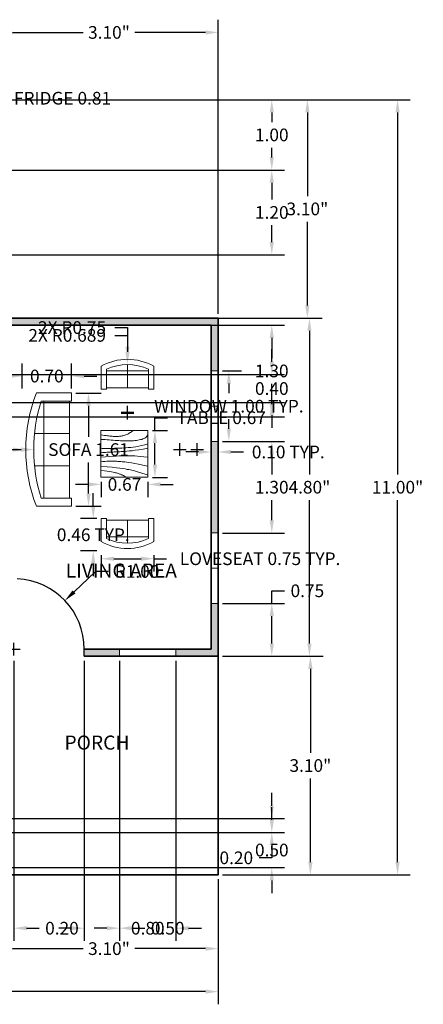
# Model space of a CAD drawing. Units: metres. Extents: x -1.9 to 13.1, y 0.9 to 14.8.
# Tile 7 of 7: x 7.4 to 13.1, y 0.9 to 14.8. Entities that reach past the tile are written whole.
import ezdxf

# ---------------------------------------------------------------- set-up
doc = ezdxf.new("R2010")
doc.units = ezdxf.units.M
doc.header["$MEASUREMENT"] = 0
for name, color, linetype, lineweight in [('A-ANNO-DIMS', 2, 'Continuous', 13), ('A-AREA-IDEN', 7, 'Continuous', 25), ('A-DOOR', 3, 'Continuous', 25), ('A-FURN', 8, 'Continuous', 18), ('A-GLAZ', 4, 'Continuous', 18), ('A-WALL', 7, 'Continuous', 35), ('A-WALL-PATT', 252, 'Continuous', 13)]:
    doc.layers.add(name, color=color, linetype=linetype, lineweight=lineweight)
doc.styles.get("Standard").update_dxf_attribs({"font": 'arial.ttf'})
doc.dimstyles.get("Standard").update_dxf_attribs({"dimtxt": 0.18, "dimasz": 0.18, "dimexe": 0.18, "dimexo": 0.0625, "dimgap": 0.09, "dimtad": 0, "dimtih": 1, "dimtoh": 1, "dimzin": 0, "dimdsep": 46, "dimlunit": 3, "dimtxsty": 'Standard', "dimcen": 0.09, "dimadec": 0, "dimazin": 0, "dimtfac": 1, "dimtofl": 0, "dimtmove": 0, "dimatfit": 3, "dimfxl": 1, "dimtolj": 1, "dimtzin": 0, "dimarcsym": 0})

# ---------------------------------------------------------------- blocks, each defined once
blk = doc.blocks.new('Table - Square Woodgrain 42 x 42 in.')
blk.add_line((0, -42), (42, -42))
for points in [[(0, -4), (1.704, -4.2172), (3.2358, -4.4188), (4.615, -4.604), (5.8615, -4.7721), (6.9951, -4.9224), (8.0357, -5.0541), (9.0031, -5.1667), (9.9171, -5.2594), (10.7951, -5.3316), (11.6445, -5.3836), (12.4702, -5.4157), (13.277, -5.4283), (14.0698, -5.4217), (14.8535, -5.3964), (15.6331, -5.3526), (16.4133, -5.2908), (17.1986, -5.2103), (17.9913, -5.1062), (18.793, -4.9727), (19.6056, -4.8038), (20.4307, -4.5937), (21.2701, -4.3365), (22.1256, -4.0262), (22.9989, -3.6571), (23.888, -3.2272), (24.7756, -2.7516), (25.6408, -2.2491), (26.4624, -1.7387), (27.2195, -1.2395), (27.891, -0.7703), (28.456, -0.3501), (28.8934, 0.002)], [(0, -42), (0, 0), (42, 0), (42, -42)], [(0, -8), (1.8203, -8.1001), (3.6741, -8.2149), (5.5411, -8.3408), (7.4011, -8.4741), (9.2339, -8.6112), (11.0193, -8.7484), (12.7371, -8.8821), (14.3671, -9.0086), (15.8954, -9.1246), (17.3337, -9.2278), (18.6997, -9.3159), (20.0116, -9.387), (21.2871, -9.4389), (22.5442, -9.4696), (23.8008, -9.477), (25.0749, -9.459), (26.3791, -9.4137), (27.7049, -9.3403), (29.0383, -9.2382), (30.3655, -9.1068), (31.6728, -8.9455), (32.9461, -8.7535), (34.1717, -8.5304), (35.3358, -8.2756), (36.4268, -7.9863), (37.443, -7.6521), (38.3849, -7.2603), (39.253, -6.7986), (40.048, -6.2542), (40.7705, -5.6147), (41.421, -4.8674), (42, -4)], [(42, -12), (39.1784, -12.8621), (36.4519, -13.5654), (33.8246, -14.1294), (31.3004, -14.5731), (28.8832, -14.9161), (26.577, -15.1775), (24.3858, -15.3768), (22.3136, -15.5332), (20.3622, -15.6632), (18.5254, -15.7718), (16.7947, -15.8612), (15.1618, -15.9338), (13.6183, -15.9916), (12.1558, -16.0369), (10.7659, -16.0718), (9.4403, -16.0987), (8.1703, -16.1191), (6.9461, -16.1325), (5.7577, -16.1377), (4.595, -16.1335), (3.4479, -16.1188), (2.3064, -16.0924), (1.1604, -16.0532), (0, -16)], [(42, -16), (37.6529, -16.7365), (33.8802, -17.329), (30.6179, -17.7961), (27.8015, -18.1561), (25.3668, -18.4275), (23.2497, -18.6288), (21.3859, -18.7785), (19.7111, -18.8949), (18.1693, -18.9939), (16.7375, -19.0795), (15.401, -19.1534), (14.1449, -19.217), (12.9544, -19.2717), (11.8148, -19.3191), (10.7113, -19.3606), (9.6291, -19.3976), (8.5534, -19.4323), (7.47, -19.4689), (6.3643, -19.5122), (5.222, -19.5672), (4.0288, -19.6386), (2.7703, -19.7313), (1.4321, -19.8501), (0, -20)], [(0, -24), (3.9243, -23.6805), (7.4766, -23.4138), (10.6891, -23.1954), (13.5943, -23.0205), (16.2247, -22.8847), (18.6125, -22.7832), (20.7903, -22.7116), (22.7903, -22.6651), (24.6563, -22.642), (26.4764, -22.6507), (28.35, -22.7024), (30.3766, -22.8084), (32.6555, -22.98), (35.2861, -23.2283), (38.3678, -23.5645), (42, -24)], [(42, -32), (37.392, -31.017), (33.4585, -30.2231), (30.1291, -29.5949), (27.3334, -29.109), (25.0009, -28.742), (23.0612, -28.4707), (21.4439, -28.2716), (20.0786, -28.1215), (18.8998, -28.0002), (17.8609, -27.9014), (16.9206, -27.8219), (16.0371, -27.7588), (15.1691, -27.709), (14.2748, -27.6693), (13.3128, -27.6368), (12.2415, -27.6083), (11.0295, -27.5824), (9.6867, -27.5643), (8.233, -27.5608), (6.6884, -27.5787), (5.0728, -27.6248), (3.4062, -27.7058), (1.7086, -27.8286), (0, -28)], [(0, -32), (5.4026, -32.5358), (9.9494, -33.019), (13.7424, -33.4553), (16.8834, -33.8505), (19.4743, -34.2106), (21.6171, -34.5413), (23.4136, -34.8486), (24.9657, -35.1382), (26.3614, -35.4156), (27.6332, -35.6841), (28.7995, -35.9467), (29.8788, -36.2064), (30.8897, -36.4661), (31.8507, -36.7288), (32.7802, -36.9973), (33.6968, -37.2747), (34.6175, -37.5635), (35.5531, -37.8651), (36.5128, -38.1805), (37.506, -38.5108), (38.5421, -38.8568), (39.6302, -39.2197), (40.7797, -39.6004), (42, -40)], [(0, -36), (3.0098, -36.2857), (5.5354, -36.5643), (7.6368, -36.8359), (9.374, -37.1009), (10.807, -37.3597), (11.9957, -37.6126), (13.0002, -37.8599), (13.8804, -38.102), (14.6874, -38.3393), (15.4365, -38.5729), (16.1338, -38.8041), (16.7858, -39.0341), (17.3987, -39.264), (17.9787, -39.4952), (18.5322, -39.7288), (19.0655, -39.9662), (19.5832, -40.2081), (20.0842, -40.4544), (20.5657, -40.7046), (21.0249, -40.9581), (21.459, -41.2144), (21.8653, -41.4731), (22.2409, -41.7335), (22.5831, -41.9951)]]:
    blk.add_lwpolyline(points)
blk = doc.blocks.new('Sofa - Roundback 7 ft.')
for p, q in [((-12.00002, -32.4421), (-12.00003, -6.5971)), ((11.99997, -32.4421), (11.99998, -6.5971)), ((-36.000027, -34), (-36.000027, -11.4696)), ((-35.999844, -13.3819), (35.9998, -13.3819)), ((35.99998, -34), (35.99998, -11.4696)), ((-36.000027, -32.4421), (35.99998, -32.4421))]:
    blk.add_line(p, q)
for points in [[(-36.000027, -34), (-42.000027, -34), (-42.000027, -8)], [(41.99998, -8), (41.99998, -34), (35.99998, -34)]]:
    blk.add_lwpolyline(points)
for centre, radius, start, end in [((0, -114.25), 114.25, 68.43141, 111.5686), ((-0.00001, -127.1968), 121.1968, 72.72033, 107.2797)]:
    blk.add_arc(centre, radius, start, end)
blk = doc.blocks.new('Sofa - Roundback Loveseat 5 ft.')
for p, q in [((0, -32.44198), (0, -5.99998)), ((-24, -33.99998), (-24, -11.46958)), ((-23.9998, -13.38178), (23.99986, -13.38178)), ((24.00004, -33.99998), (24.00004, -11.46958)), ((-24, -32.44198), (24.00004, -32.44198))]:
    blk.add_line(p, q)
for points in [[(-24, -33.99998), (-30, -33.99998), (-30, -7.99998)], [(30.00004, -7.99998), (30.00004, -33.99998), (24.00004, -33.99998)]]:
    blk.add_lwpolyline(points)
for centre, radius, start, end in [((0, -60.24998), 60.24998, 60.13715, 119.8628), ((0, -61.38438), 55.38444, 64.32083, 115.6792)]:
    blk.add_arc(centre, radius, start, end)
blk = doc.blocks.new('*D11')
at = {"layer": 'A-ANNO-DIMS', "color": 0, "lineweight": -2, "transparency": 16777216}
for p, q in [((7.104, 2.634), (7.104, 1.467)), ((10.204, 2.634), (10.204, 1.467)), ((7.284, 1.647), (8.286, 1.647)), ((10.024, 1.647), (9.022, 1.647))]:
    blk.add_line(p, q, dxfattribs=at)
at = {"layer": 'A-ANNO-DIMS', "color": 0, "transparency": 16777216}
for points in [[(7.284, 1.677), (7.284, 1.617), (7.104, 1.647)], [(10.024, 1.677), (10.024, 1.617), (10.204, 1.647)]]:
    blk.add_solid(points, dxfattribs=at)
at = {"layer": 'Defpoints', "color": 0, "transparency": 16777216}
for p in [(7.104, 2.696), (10.204, 2.696), (10.204, 1.647)]:
    blk.add_point(p, dxfattribs=at)
at = {"layer": 'A-ANNO-DIMS', "color": 0, "transparency": 16777216, "insert": (8.654, 1.647), "char_height": 0.18, "attachment_point": 5}
blk.add_mtext('\\A1;3.10"', dxfattribs=at)
blk = doc.blocks.new('*D12')
at = {"layer": 'A-ANNO-DIMS', "color": 0, "lineweight": -2, "transparency": 16777216}
for p, q in [((1.204, 2.634), (1.204, 0.857)), ((10.204, 2.634), (10.204, 0.857)), ((1.384, 1.037), (5.336, 1.037)), ((10.024, 1.037), (6.072, 1.037))]:
    blk.add_line(p, q, dxfattribs=at)
at = {"layer": 'A-ANNO-DIMS', "color": 0, "transparency": 16777216}
for points in [[(1.384, 1.067), (1.384, 1.007), (1.204, 1.037)], [(10.024, 1.067), (10.024, 1.007), (10.204, 1.037)]]:
    blk.add_solid(points, dxfattribs=at)
at = {"layer": 'Defpoints', "color": 0, "transparency": 16777216}
for p in [(1.204, 2.696), (10.204, 2.696), (10.204, 1.037)]:
    blk.add_point(p, dxfattribs=at)
at = {"layer": 'A-ANNO-DIMS', "color": 0, "transparency": 16777216, "insert": (5.704, 1.037), "char_height": 0.18, "attachment_point": 5}
blk.add_mtext('\\A1;9.00"', dxfattribs=at)
blk = doc.blocks.new('*D13')
at = {"layer": 'A-ANNO-DIMS', "color": 0, "lineweight": -2, "transparency": 16777216}
for p, q in [((7.166, 13.696), (12.927, 13.696)), ((12.747, 13.516), (12.747, 8.378)), ((12.747, 2.876), (12.747, 8.014)), ((10.266, 2.696), (12.927, 2.696))]:
    blk.add_line(p, q, dxfattribs=at)
at = {"layer": 'A-ANNO-DIMS', "color": 0, "transparency": 16777216}
for points in [[(12.717, 13.516), (12.777, 13.516), (12.747, 13.696)], [(12.717, 2.876), (12.777, 2.876), (12.747, 2.696)]]:
    blk.add_solid(points, dxfattribs=at)
at = {"layer": 'Defpoints', "color": 0, "transparency": 16777216}
for p in [(7.104, 13.696), (12.747, 13.696), (10.204, 2.696)]:
    blk.add_point(p, dxfattribs=at)
at = {"layer": 'A-ANNO-DIMS', "color": 0, "transparency": 16777216, "insert": (12.747, 8.196), "char_height": 0.18, "attachment_point": 5}
blk.add_mtext('\\A1;11.00"', dxfattribs=at)
blk = doc.blocks.new('*D14')
at = {"layer": 'A-ANNO-DIMS', "color": 0, "lineweight": -2, "transparency": 16777216}
for p, q in [((10.266, 5.796), (11.691, 5.796)), ((11.511, 5.616), (11.511, 4.428)), ((11.511, 2.876), (11.511, 4.064)), ((10.266, 2.696), (11.691, 2.696))]:
    blk.add_line(p, q, dxfattribs=at)
at = {"layer": 'A-ANNO-DIMS', "color": 0, "transparency": 16777216}
for points in [[(11.481, 5.616), (11.541, 5.616), (11.511, 5.796)], [(11.481, 2.876), (11.541, 2.876), (11.511, 2.696)]]:
    blk.add_solid(points, dxfattribs=at)
at = {"layer": 'Defpoints', "color": 0, "transparency": 16777216}
for p in [(10.204, 5.796), (11.511, 5.796), (10.204, 2.696)]:
    blk.add_point(p, dxfattribs=at)
at = {"layer": 'A-ANNO-DIMS', "color": 0, "transparency": 16777216, "insert": (11.511, 4.246), "char_height": 0.18, "attachment_point": 5}
blk.add_mtext('\\A1;3.10"', dxfattribs=at)
blk = doc.blocks.new('*D15')
at = {"layer": 'A-ANNO-DIMS', "color": 0, "lineweight": -2, "transparency": 16777216}
for p, q in [((10.266, 10.596), (11.677, 10.596)), ((11.497, 10.416), (11.497, 8.378)), ((11.497, 5.976), (11.497, 8.014)), ((10.266, 5.796), (11.677, 5.796))]:
    blk.add_line(p, q, dxfattribs=at)
at = {"layer": 'A-ANNO-DIMS', "color": 0, "transparency": 16777216}
for points in [[(11.467, 10.416), (11.527, 10.416), (11.497, 10.596)], [(11.467, 5.976), (11.527, 5.976), (11.497, 5.796)]]:
    blk.add_solid(points, dxfattribs=at)
at = {"layer": 'Defpoints', "color": 0, "transparency": 16777216}
for p in [(10.204, 10.596), (11.497, 10.596), (10.204, 5.796)]:
    blk.add_point(p, dxfattribs=at)
at = {"layer": 'A-ANNO-DIMS', "color": 0, "transparency": 16777216, "insert": (11.497, 8.196), "char_height": 0.18, "attachment_point": 5}
blk.add_mtext('\\A1;4.80"', dxfattribs=at)
blk = doc.blocks.new('*D16')
at = {"layer": 'A-ANNO-DIMS', "color": 0, "lineweight": -2, "transparency": 16777216}
for p, q in [((7.166, 13.696), (11.648, 13.696)), ((11.468, 13.516), (11.468, 12.328)), ((11.468, 10.776), (11.468, 11.964)), ((7.166, 10.596), (11.648, 10.596))]:
    blk.add_line(p, q, dxfattribs=at)
at = {"layer": 'A-ANNO-DIMS', "color": 0, "transparency": 16777216}
for points in [[(11.438, 13.516), (11.498, 13.516), (11.468, 13.696)], [(11.438, 10.776), (11.498, 10.776), (11.468, 10.596)]]:
    blk.add_solid(points, dxfattribs=at)
at = {"layer": 'Defpoints', "color": 0, "transparency": 16777216}
for p in [(7.104, 13.696), (11.468, 13.696), (7.104, 10.596)]:
    blk.add_point(p, dxfattribs=at)
at = {"layer": 'A-ANNO-DIMS', "color": 0, "transparency": 16777216, "insert": (11.468, 12.146), "char_height": 0.18, "attachment_point": 5}
blk.add_mtext('\\A1;3.10"', dxfattribs=at)
blk = doc.blocks.new('*D17')
at = {"layer": 'A-ANNO-DIMS', "color": 0, "lineweight": -2, "transparency": 16777216}
for p, q in [((7.104, 13.759), (7.104, 14.831)), ((10.204, 10.659), (10.204, 14.831)), ((7.284, 14.651), (8.286, 14.651)), ((10.024, 14.651), (9.022, 14.651))]:
    blk.add_line(p, q, dxfattribs=at)
at = {"layer": 'A-ANNO-DIMS', "color": 0, "transparency": 16777216}
for points in [[(7.284, 14.681), (7.284, 14.621), (7.104, 14.651)], [(10.024, 14.681), (10.024, 14.621), (10.204, 14.651)]]:
    blk.add_solid(points, dxfattribs=at)
at = {"layer": 'Defpoints', "color": 0, "transparency": 16777216}
for p in [(7.104, 14.651), (7.104, 13.696), (10.204, 10.596)]:
    blk.add_point(p, dxfattribs=at)
at = {"layer": 'A-ANNO-DIMS', "color": 0, "transparency": 16777216, "insert": (8.654, 14.651), "char_height": 0.18, "attachment_point": 5}
blk.add_mtext('\\A1;3.10"', dxfattribs=at)
blk = doc.blocks.new('WIN-1000')
for p, q in [((0.1, 1), (0, 1)), ((0.1, 0.5), (0, 0.5)), ((0.1, 0), (0, 0))]:
    blk.add_line(p, q)
blk = doc.blocks.new('*D28')
at = {"layer": 'A-ANNO-DIMS', "color": 0, "lineweight": -2, "transparency": 16777216}
for p, q in [((10.266, 9.846), (10.534, 9.846)), ((10.354, 9.666), (10.354, 9.53)), ((10.354, 9.026), (10.354, 9.163)), ((10.266, 8.846), (10.534, 8.846))]:
    blk.add_line(p, q, dxfattribs=at)
at = {"layer": 'A-ANNO-DIMS', "color": 0, "transparency": 16777216}
for points in [[(10.324, 9.666), (10.384, 9.666), (10.354, 9.846)], [(10.324, 9.026), (10.384, 9.026), (10.354, 8.846)]]:
    blk.add_solid(points, dxfattribs=at)
at = {"layer": 'Defpoints', "color": 0, "transparency": 16777216}
for p in [(10.204, 9.846), (10.354, 9.846), (10.204, 8.846)]:
    blk.add_point(p, dxfattribs=at)
at = {"layer": 'A-ANNO-DIMS', "color": 0, "transparency": 16777216, "insert": (10.354, 9.346), "char_height": 0.18, "attachment_point": 5}
blk.add_mtext('\\A1;WINDOW 1.00 TYP.', dxfattribs=at)
blk = doc.blocks.new('*D29')
at = {"layer": 'A-ANNO-DIMS', "color": 0, "lineweight": -2, "transparency": 16777216}
for p, q in [((9.924, 8.696), (9.744, 8.696)), ((10.104, 8.784), (10.104, 8.516)), ((10.204, 8.784), (10.204, 8.516)), ((10.384, 8.696), (10.564, 8.696))]:
    blk.add_line(p, q, dxfattribs=at)
at = {"layer": 'A-ANNO-DIMS', "color": 0, "transparency": 16777216}
for points in [[(9.924, 8.726), (9.924, 8.666), (10.104, 8.696)], [(10.384, 8.726), (10.384, 8.666), (10.204, 8.696)]]:
    blk.add_solid(points, dxfattribs=at)
at = {"layer": 'Defpoints', "color": 0, "transparency": 16777216}
for p in [(10.104, 8.846), (10.204, 8.846), (10.204, 8.696)]:
    blk.add_point(p, dxfattribs=at)
at = {"layer": 'A-ANNO-DIMS', "color": 0, "transparency": 16777216, "insert": (11.197, 8.696), "char_height": 0.18, "attachment_point": 5}
blk.add_mtext('\\A1;0.10 TYP.', dxfattribs=at)
blk = doc.blocks.new('*D38')
at = {"layer": 'A-ANNO-DIMS', "color": 0, "lineweight": -2, "transparency": 16777216}
for p, q in [((8.543, 7.231), (8.543, 7.001)), ((8.723, 7.181), (9.11, 7.181)), ((9.29, 7.231), (9.29, 7.001)), ((9.29, 7.181), (9.47, 7.181))]:
    blk.add_line(p, q, dxfattribs=at)
at = {"layer": 'A-ANNO-DIMS', "color": 0, "transparency": 16777216}
for points in [[(8.723, 7.211), (8.723, 7.151), (8.543, 7.181)], [(9.11, 7.211), (9.11, 7.151), (9.29, 7.181)]]:
    blk.add_solid(points, dxfattribs=at)
at = {"layer": 'Defpoints', "color": 0, "transparency": 16777216}
for p in [(8.543, 7.293), (9.29, 7.293), (9.29, 7.181)]:
    blk.add_point(p, dxfattribs=at)
at = {"layer": 'A-ANNO-DIMS', "color": 0, "transparency": 16777216, "insert": (10.797, 7.181), "char_height": 0.18, "attachment_point": 5}
blk.add_mtext('\\A1;LOVESEAT 0.75 TYP.', dxfattribs=at)
blk = doc.blocks.new('*D39')
at = {"layer": 'A-ANNO-DIMS', "color": 0, "lineweight": -2, "transparency": 16777216}
for p, q in [((8.431, 7.93), (8.431, 8.11)), ((8.481, 7.75), (8.251, 7.75)), ((8.481, 7.293), (8.251, 7.293)), ((8.431, 7.113), (8.431, 6.933))]:
    blk.add_line(p, q, dxfattribs=at)
at = {"layer": 'A-ANNO-DIMS', "color": 0, "transparency": 16777216}
for points in [[(8.401, 7.93), (8.461, 7.93), (8.431, 7.75)], [(8.401, 7.113), (8.461, 7.113), (8.431, 7.293)]]:
    blk.add_solid(points, dxfattribs=at)
at = {"layer": 'Defpoints', "color": 0, "transparency": 16777216}
for p in [(8.543, 7.75), (8.431, 7.293), (8.543, 7.293)]:
    blk.add_point(p, dxfattribs=at)
at = {"layer": 'A-ANNO-DIMS', "color": 0, "transparency": 16777216, "insert": (8.431, 7.521), "char_height": 0.18, "attachment_point": 5}
blk.add_mtext('\\A1;0.46 TYP.', dxfattribs=at)
blk = doc.blocks.new('*D40')
at = {"layer": 'A-ANNO-DIMS', "color": 0, "lineweight": -2, "transparency": 16777216}
for p, q in [((9.306, 9.002), (9.306, 9.182)), ((9.306, 9.182), (9.486, 9.182)), ((9.269, 9.002), (9.486, 9.002)), ((9.306, 8.516), (9.306, 8.822)), ((9.269, 8.336), (9.486, 8.336))]:
    blk.add_line(p, q, dxfattribs=at)
at = {"layer": 'A-ANNO-DIMS', "color": 0, "transparency": 16777216}
for points in [[(9.276, 8.822), (9.336, 8.822), (9.306, 9.002)], [(9.276, 8.516), (9.336, 8.516), (9.306, 8.336)]]:
    blk.add_solid(points, dxfattribs=at)
at = {"layer": 'Defpoints', "color": 0, "transparency": 16777216}
for p in [(9.206, 9.002), (9.306, 9.002), (9.206, 8.336)]:
    blk.add_point(p, dxfattribs=at)
at = {"layer": 'A-ANNO-DIMS', "color": 0, "transparency": 16777216, "insert": (10.246, 9.182), "char_height": 0.18, "attachment_point": 5}
blk.add_mtext('\\A1;TABLE 0.67', dxfattribs=at)
blk = doc.blocks.new('*D41')
at = {"layer": 'A-ANNO-DIMS', "color": 0, "lineweight": -2, "transparency": 16777216}
for p, q in [((8.541, 8.274), (8.541, 8.056)), ((9.206, 8.274), (9.206, 8.056)), ((8.361, 8.236), (8.181, 8.236)), ((9.386, 8.236), (9.566, 8.236))]:
    blk.add_line(p, q, dxfattribs=at)
at = {"layer": 'A-ANNO-DIMS', "color": 0, "transparency": 16777216}
for points in [[(8.361, 8.266), (8.361, 8.206), (8.541, 8.236)], [(9.386, 8.266), (9.386, 8.206), (9.206, 8.236)]]:
    blk.add_solid(points, dxfattribs=at)
at = {"layer": 'Defpoints', "color": 0, "transparency": 16777216}
for p in [(8.541, 8.336), (9.206, 8.336), (9.206, 8.236)]:
    blk.add_point(p, dxfattribs=at)
at = {"layer": 'A-ANNO-DIMS', "color": 0, "transparency": 16777216, "insert": (8.874, 8.236), "char_height": 0.18, "attachment_point": 5}
blk.add_mtext('\\A1;0.67', dxfattribs=at)
blk = doc.blocks.new('*D42')
at = {"layer": 'A-ANNO-DIMS', "color": 0, "lineweight": -2, "transparency": 16777216}
for p, q in [((8.185, 9.533), (8.544, 9.533)), ((8.364, 9.353), (8.364, 8.913)), ((8.364, 8.106), (8.364, 8.547)), ((8.185, 7.926), (8.544, 7.926))]:
    blk.add_line(p, q, dxfattribs=at)
at = {"layer": 'A-ANNO-DIMS', "color": 0, "transparency": 16777216}
for points in [[(8.334, 9.353), (8.394, 9.353), (8.364, 9.533)], [(8.334, 8.106), (8.394, 8.106), (8.364, 7.926)]]:
    blk.add_solid(points, dxfattribs=at)
at = {"layer": 'Defpoints', "color": 0, "transparency": 16777216}
for p in [(8.123, 9.533), (8.364, 9.533), (8.123, 7.926)]:
    blk.add_point(p, dxfattribs=at)
at = {"layer": 'A-ANNO-DIMS', "color": 0, "transparency": 16777216, "insert": (8.364, 8.73), "char_height": 0.18, "attachment_point": 5}
blk.add_mtext('\\A1;SOFA 1.61', dxfattribs=at)
blk = doc.blocks.new('*D43')
at = {"layer": 'A-ANNO-DIMS', "color": 0, "lineweight": -2, "transparency": 16777216}
for p, q in [((7.421, 9.596), (7.421, 9.954)), ((8.123, 9.596), (8.123, 9.954)), ((7.241, 9.774), (7.061, 9.774)), ((8.303, 9.774), (8.483, 9.774))]:
    blk.add_line(p, q, dxfattribs=at)
at = {"layer": 'A-ANNO-DIMS', "color": 0, "transparency": 16777216}
for points in [[(7.241, 9.804), (7.241, 9.744), (7.421, 9.774)], [(8.303, 9.804), (8.303, 9.744), (8.123, 9.774)]]:
    blk.add_solid(points, dxfattribs=at)
at = {"layer": 'Defpoints', "color": 0, "transparency": 16777216}
for p in [(7.421, 9.774), (7.421, 9.533), (8.123, 9.533)]:
    blk.add_point(p, dxfattribs=at)
at = {"layer": 'A-ANNO-DIMS', "color": 0, "transparency": 16777216, "insert": (7.772, 9.774), "char_height": 0.18, "attachment_point": 5}
blk.add_mtext('\\A1;0.70', dxfattribs=at)
blk = doc.blocks.new('*D46')
at = {"layer": 'A-ANNO-DIMS', "color": 0, "lineweight": -2, "transparency": 16777216}
for p, q in [((6.197, 13.659), (6.197, 13.897)), ((7.004, 13.659), (7.004, 13.897)), ((6.377, 13.717), (6.824, 13.717)), ((7.004, 13.717), (7.184, 13.717))]:
    blk.add_line(p, q, dxfattribs=at)
at = {"layer": 'A-ANNO-DIMS', "color": 0, "transparency": 16777216}
for points in [[(6.377, 13.747), (6.377, 13.687), (6.197, 13.717)], [(6.824, 13.747), (6.824, 13.687), (7.004, 13.717)]]:
    blk.add_solid(points, dxfattribs=at)
at = {"layer": 'Defpoints', "color": 0, "transparency": 16777216}
for p in [(7.004, 13.717), (6.197, 13.596), (7.004, 13.596)]:
    blk.add_point(p, dxfattribs=at)
at = {"layer": 'A-ANNO-DIMS', "color": 0, "transparency": 16777216, "insert": (7.995, 13.717), "char_height": 0.18, "attachment_point": 5}
blk.add_mtext('\\A1;FRIDGE 0.81', dxfattribs=at)
blk = doc.blocks.new('*D55')
at = {"layer": 'A-ANNO-DIMS', "color": 0, "lineweight": -2, "transparency": 16777216}
for p, q in [((10.963, 6.546), (10.963, 6.726)), ((10.963, 6.726), (11.143, 6.726)), ((10.266, 6.546), (11.143, 6.546)), ((10.963, 5.976), (10.963, 6.366)), ((10.266, 5.796), (11.143, 5.796))]:
    blk.add_line(p, q, dxfattribs=at)
at = {"layer": 'A-ANNO-DIMS', "color": 0, "transparency": 16777216}
for points in [[(10.933, 6.366), (10.993, 6.366), (10.963, 6.546)], [(10.933, 5.976), (10.993, 5.976), (10.963, 5.796)]]:
    blk.add_solid(points, dxfattribs=at)
at = {"layer": 'Defpoints', "color": 0, "transparency": 16777216}
for p in [(10.204, 6.546), (10.963, 6.546), (10.204, 5.796)]:
    blk.add_point(p, dxfattribs=at)
at = {"layer": 'A-ANNO-DIMS', "color": 0, "transparency": 16777216, "insert": (11.468, 6.726), "char_height": 0.18, "attachment_point": 5}
blk.add_mtext('\\A1;0.75', dxfattribs=at)
blk = doc.blocks.new('*D56')
at = {"layer": 'A-ANNO-DIMS', "color": 0, "lineweight": -2, "transparency": 16777216}
for p, q in [((10.266, 8.846), (11.143, 8.846)), ((10.963, 8.666), (10.963, 8.378)), ((10.963, 7.726), (10.963, 8.014)), ((10.266, 7.546), (11.143, 7.546))]:
    blk.add_line(p, q, dxfattribs=at)
at = {"layer": 'A-ANNO-DIMS', "color": 0, "transparency": 16777216}
for points in [[(10.933, 8.666), (10.993, 8.666), (10.963, 8.846)], [(10.933, 7.726), (10.993, 7.726), (10.963, 7.546)]]:
    blk.add_solid(points, dxfattribs=at)
at = {"layer": 'Defpoints', "color": 0, "transparency": 16777216}
for p in [(10.204, 8.846), (10.963, 8.846), (10.204, 7.546)]:
    blk.add_point(p, dxfattribs=at)
at = {"layer": 'A-ANNO-DIMS', "color": 0, "transparency": 16777216, "insert": (10.963, 8.196), "char_height": 0.18, "attachment_point": 5}
blk.add_mtext('\\A1;1.30', dxfattribs=at)
blk = doc.blocks.new('*D57')
at = {"layer": 'A-ANNO-DIMS', "color": 0, "lineweight": -2, "transparency": 16777216}
for p, q in [((8.304, 5.734), (8.304, 1.757)), ((8.804, 5.734), (8.804, 1.757)), ((8.124, 1.937), (7.944, 1.937)), ((8.984, 1.937), (9.164, 1.937))]:
    blk.add_line(p, q, dxfattribs=at)
at = {"layer": 'A-ANNO-DIMS', "color": 0, "transparency": 16777216}
for points in [[(8.124, 1.967), (8.124, 1.907), (8.304, 1.937)], [(8.984, 1.967), (8.984, 1.907), (8.804, 1.937)]]:
    blk.add_solid(points, dxfattribs=at)
at = {"layer": 'Defpoints', "color": 0, "transparency": 16777216}
for p in [(8.304, 5.796), (8.804, 5.796), (8.804, 1.937)]:
    blk.add_point(p, dxfattribs=at)
at = {"layer": 'A-ANNO-DIMS', "color": 0, "transparency": 16777216, "insert": (9.487, 1.937), "char_height": 0.18, "attachment_point": 5}
blk.add_mtext('\\A1;0.50', dxfattribs=at)
blk = doc.blocks.new('*D58')
at = {"layer": 'A-ANNO-DIMS', "color": 0, "lineweight": -2, "transparency": 16777216}
for p, q in [((8.803847, 5.733878), (8.803847, 1.756878)), ((9.603847, 5.733878), (9.603847, 1.756878)), ((8.623847, 1.936878), (8.443847, 1.936878)), ((9.783847, 1.936878), (9.963847, 1.936878))]:
    blk.add_line(p, q, dxfattribs=at)
at = {"layer": 'A-ANNO-DIMS', "color": 0, "transparency": 16777216}
for points in [[(8.623847, 1.966878), (8.623847, 1.906878), (8.803847, 1.936878)], [(9.783847, 1.966878), (9.783847, 1.906878), (9.603847, 1.936878)]]:
    blk.add_solid(points, dxfattribs=at)
at = {"layer": 'Defpoints', "color": 0, "transparency": 16777216}
for p in [(8.803847, 5.796378), (9.603847, 5.796378), (8.803847, 1.936878)]:
    blk.add_point(p, dxfattribs=at)
at = {"layer": 'A-ANNO-DIMS', "color": 0, "transparency": 16777216, "insert": (9.203847, 1.936878), "char_height": 0.18, "attachment_point": 5}
blk.add_mtext('\\A1;0.80', dxfattribs=at)
blk = doc.blocks.new('*D59')
at = {"layer": 'A-ANNO-DIMS', "color": 0, "lineweight": -2, "transparency": 16777216}
for p, q in [((7.104, 5.734), (7.104, 1.757)), ((7.304, 5.734), (7.304, 1.757)), ((6.924, 1.937), (6.744, 1.937)), ((7.484, 1.937), (7.664, 1.937))]:
    blk.add_line(p, q, dxfattribs=at)
at = {"layer": 'A-ANNO-DIMS', "color": 0, "transparency": 16777216}
for points in [[(6.924, 1.967), (6.924, 1.907), (7.104, 1.937)], [(7.484, 1.967), (7.484, 1.907), (7.304, 1.937)]]:
    blk.add_solid(points, dxfattribs=at)
at = {"layer": 'Defpoints', "color": 0, "transparency": 16777216}
for p in [(7.104, 5.796), (7.304, 5.796), (7.304, 1.937)]:
    blk.add_point(p, dxfattribs=at)
at = {"layer": 'A-ANNO-DIMS', "color": 0, "transparency": 16777216, "insert": (7.987, 1.937), "char_height": 0.18, "attachment_point": 5}
blk.add_mtext('\\A1;0.20', dxfattribs=at)
blk = doc.blocks.new('*D60')
at = {"layer": 'A-ANNO-DIMS', "color": 0, "lineweight": -2, "transparency": 16777216}
for p, q in [((7.166, 13.696), (11.143, 13.696)), ((10.963, 13.516), (10.963, 13.378)), ((10.963, 12.876), (10.963, 13.014)), ((7.166, 12.696), (11.143, 12.696))]:
    blk.add_line(p, q, dxfattribs=at)
at = {"layer": 'A-ANNO-DIMS', "color": 0, "transparency": 16777216}
for points in [[(10.933, 13.516), (10.993, 13.516), (10.963, 13.696)], [(10.933, 12.876), (10.993, 12.876), (10.963, 12.696)]]:
    blk.add_solid(points, dxfattribs=at)
at = {"layer": 'Defpoints', "color": 0, "transparency": 16777216}
for p in [(7.104, 13.696), (10.963, 13.696), (7.104, 12.696)]:
    blk.add_point(p, dxfattribs=at)
at = {"layer": 'A-ANNO-DIMS', "color": 0, "transparency": 16777216, "insert": (10.963, 13.196), "char_height": 0.18, "attachment_point": 5}
blk.add_mtext('\\A1;1.00', dxfattribs=at)
blk = doc.blocks.new('*D61')
at = {"layer": 'A-ANNO-DIMS', "color": 0, "lineweight": -2, "transparency": 16777216}
for p, q in [((7.166, 12.696), (11.143, 12.696)), ((10.963, 12.516), (10.963, 12.278)), ((10.963, 11.676), (10.963, 11.914)), ((7.166, 11.496), (11.143, 11.496))]:
    blk.add_line(p, q, dxfattribs=at)
at = {"layer": 'A-ANNO-DIMS', "color": 0, "transparency": 16777216}
for points in [[(10.933, 12.516), (10.993, 12.516), (10.963, 12.696)], [(10.933, 11.676), (10.993, 11.676), (10.963, 11.496)]]:
    blk.add_solid(points, dxfattribs=at)
at = {"layer": 'Defpoints', "color": 0, "transparency": 16777216}
for p in [(7.104, 12.696), (7.104, 11.496), (10.963, 11.496)]:
    blk.add_point(p, dxfattribs=at)
at = {"layer": 'A-ANNO-DIMS', "color": 0, "transparency": 16777216, "insert": (10.963, 12.096), "char_height": 0.18, "attachment_point": 5}
blk.add_mtext('\\A1;1.20', dxfattribs=at)
blk = doc.blocks.new('*D65')
at = {"layer": 'A-ANNO-DIMS', "color": 0, "lineweight": -2, "transparency": 16777216}
for p, q in [((10.963347, 9.976378), (10.963347, 10.156378)), ((2.966347, 9.796378), (11.143347, 9.796378)), ((2.966347, 9.396378), (11.143347, 9.396378)), ((10.963347, 9.216378), (10.963347, 9.036378))]:
    blk.add_line(p, q, dxfattribs=at)
at = {"layer": 'A-ANNO-DIMS', "color": 0, "transparency": 16777216}
for points in [[(10.933347, 9.976378), (10.993347, 9.976378), (10.963347, 9.796378)], [(10.933347, 9.216378), (10.993347, 9.216378), (10.963347, 9.396378)]]:
    blk.add_solid(points, dxfattribs=at)
at = {"layer": 'Defpoints', "color": 0, "transparency": 16777216}
for p in [(2.903847, 9.796378), (2.903847, 9.396378), (10.963347, 9.396378)]:
    blk.add_point(p, dxfattribs=at)
at = {"layer": 'A-ANNO-DIMS', "color": 0, "transparency": 16777216, "insert": (10.963347, 9.596378), "char_height": 0.18, "attachment_point": 5}
blk.add_mtext('\\A1;0.40', dxfattribs=at)
blk = doc.blocks.new('*D67')
at = {"layer": 'A-ANNO-DIMS', "color": 0, "lineweight": -2, "transparency": 16777216}
for p, q in [((10.963, 3.676), (10.963, 3.856)), ((7.066, 3.496), (11.143, 3.496)), ((7.066, 3.296), (11.143, 3.296)), ((10.963, 3.116), (10.963, 2.936)), ((10.963, 2.936), (10.783, 2.936))]:
    blk.add_line(p, q, dxfattribs=at)
at = {"layer": 'A-ANNO-DIMS', "color": 0, "transparency": 16777216}
for points in [[(10.933, 3.676), (10.993, 3.676), (10.963, 3.496)], [(10.933, 3.116), (10.993, 3.116), (10.963, 3.296)]]:
    blk.add_solid(points, dxfattribs=at)
at = {"layer": 'Defpoints', "color": 0, "transparency": 16777216}
for p in [(7.004, 3.496), (7.004, 3.296), (10.963, 3.296)]:
    blk.add_point(p, dxfattribs=at)
at = {"layer": 'A-ANNO-DIMS', "color": 0, "transparency": 16777216, "insert": (10.46, 2.936), "char_height": 0.18, "attachment_point": 5}
blk.add_mtext('\\A1;0.20', dxfattribs=at)
blk = doc.blocks.new('*D68')
at = {"layer": 'A-ANNO-DIMS', "color": 0, "lineweight": -2, "transparency": 16777216}
for p, q in [((10.963347, 3.476378), (10.963347, 3.656378)), ((7.066347, 3.296378), (11.143347, 3.296378)), ((7.066347, 2.796378), (11.143347, 2.796378)), ((10.963347, 2.616378), (10.963347, 2.436378))]:
    blk.add_line(p, q, dxfattribs=at)
at = {"layer": 'A-ANNO-DIMS', "color": 0, "transparency": 16777216}
for points in [[(10.933347, 3.476378), (10.993347, 3.476378), (10.963347, 3.296378)], [(10.933347, 2.616378), (10.993347, 2.616378), (10.963347, 2.796378)]]:
    blk.add_solid(points, dxfattribs=at)
at = {"layer": 'Defpoints', "color": 0, "transparency": 16777216}
for p in [(7.003847, 3.296378), (7.003847, 2.796378), (10.963347, 2.796378)]:
    blk.add_point(p, dxfattribs=at)
at = {"layer": 'A-ANNO-DIMS', "color": 0, "transparency": 16777216, "insert": (10.963347, 3.046378), "char_height": 0.18, "attachment_point": 5}
blk.add_mtext('\\A1;0.50', dxfattribs=at)
blk = doc.blocks.new('*D74')
at = {"layer": 'A-ANNO-DIMS', "color": 0, "lineweight": -2, "transparency": 16777216}
for p, q in [((7.166, 10.496), (11.143, 10.496)), ((10.963, 10.316), (10.963, 10.028)), ((10.963, 9.376), (10.963, 9.664)), ((7.166, 9.196), (11.143, 9.196))]:
    blk.add_line(p, q, dxfattribs=at)
at = {"layer": 'A-ANNO-DIMS', "color": 0, "transparency": 16777216}
for points in [[(10.933, 10.316), (10.993, 10.316), (10.963, 10.496)], [(10.933, 9.376), (10.993, 9.376), (10.963, 9.196)]]:
    blk.add_solid(points, dxfattribs=at)
at = {"layer": 'Defpoints', "color": 0, "transparency": 16777216}
for p in [(7.104, 10.496), (10.963, 10.496), (7.104, 9.196)]:
    blk.add_point(p, dxfattribs=at)
at = {"layer": 'A-ANNO-DIMS', "color": 0, "transparency": 16777216, "insert": (10.963, 9.846), "char_height": 0.18, "attachment_point": 5}
blk.add_mtext('\\A1;1.30', dxfattribs=at)
blk = doc.blocks.new('*D75')
at = {"layer": 'A-ANNO-DIMS', "color": 0, "lineweight": -2, "transparency": 16777216}
for p, q in [((8.464, 7), (8.159, 6.71)), ((8.644, 7), (8.464, 7)), ((7.213, 5.896), (7.393, 5.896)), ((7.303, 5.806), (7.303, 5.986))]:
    blk.add_line(p, q, dxfattribs=at)
at = {"layer": 'A-ANNO-DIMS', "color": 0, "transparency": 16777216}
blk.add_solid([(8.138, 6.732), (8.179, 6.689), (8.028, 6.586)], dxfattribs=at)
at = {"layer": 'Defpoints', "color": 0, "transparency": 16777216}
for p in [(8.028, 6.586), (7.303, 5.896)]:
    blk.add_point(p, dxfattribs=at)
at = {"layer": 'A-ANNO-DIMS', "color": 0, "transparency": 16777216, "insert": (9.053, 7), "char_height": 0.18, "attachment_point": 5}
blk.add_mtext('\\A1;R1.00', dxfattribs=at)
blk = doc.blocks.new('*D78')
at = {"layer": 'A-ANNO-DIMS', "color": 0, "lineweight": -2, "transparency": 16777216}
for p, q in [((9.906, 8.64), (9.906, 8.82)), ((6.196, 8.73), (7.407, 8.73)), ((9.816, 8.73), (9.996, 8.73))]:
    blk.add_line(p, q, dxfattribs=at)
at = {"layer": 'A-ANNO-DIMS', "color": 0, "transparency": 16777216}
blk.add_solid([(7.407, 8.76), (7.407, 8.7), (7.587, 8.73)], dxfattribs=at)
at = {"layer": 'Defpoints', "color": 0, "transparency": 16777216}
for p in [(7.587, 8.73), (9.906, 8.73)]:
    blk.add_point(p, dxfattribs=at)
at = {"layer": 'A-ANNO-DIMS', "color": 0, "transparency": 16777216, "insert": (5.787, 8.73), "char_height": 0.18, "attachment_point": 5}
blk.add_mtext('\\A1;R2.32', dxfattribs=at)
blk = doc.blocks.new('*D79')
at = {"layer": 'A-ANNO-DIMS', "color": 0, "lineweight": -2, "transparency": 16777216}
for p, q in [((9.658, 8.64), (9.658, 8.82)), ((6.161, 8.73), (7.292, 8.73)), ((9.568, 8.73), (9.748, 8.73))]:
    blk.add_line(p, q, dxfattribs=at)
at = {"layer": 'A-ANNO-DIMS', "color": 0, "transparency": 16777216}
blk.add_solid([(7.292, 8.76), (7.292, 8.7), (7.472, 8.73)], dxfattribs=at)
at = {"layer": 'Defpoints', "color": 0, "transparency": 16777216}
for p in [(7.472, 8.73), (9.658, 8.73)]:
    blk.add_point(p, dxfattribs=at)
at = {"layer": 'A-ANNO-DIMS', "color": 0, "transparency": 16777216, "insert": (5.751, 8.73), "char_height": 0.18, "attachment_point": 5}
blk.add_mtext('\\A1;R2.19', dxfattribs=at)
blk = doc.blocks.new('*D80')
at = {"layer": 'A-ANNO-DIMS', "color": 0, "lineweight": -2, "transparency": 16777216}
for p, q in [((8.736, 10.462), (8.916, 10.462)), ((8.916, 10.462), (8.916, 10.192)), ((8.826, 9.262), (9.006, 9.262)), ((8.916, 9.172), (8.916, 9.352))]:
    blk.add_line(p, q, dxfattribs=at)
at = {"layer": 'A-ANNO-DIMS', "color": 0, "transparency": 16777216}
blk.add_solid([(8.946, 10.192), (8.886, 10.192), (8.916, 10.012)], dxfattribs=at)
at = {"layer": 'Defpoints', "color": 0, "transparency": 16777216}
for p in [(8.916, 10.012), (8.916, 9.262)]:
    blk.add_point(p, dxfattribs=at)
at = {"layer": 'A-ANNO-DIMS', "color": 0, "transparency": 16777216, "insert": (8.13, 10.462), "char_height": 0.18, "attachment_point": 5}
blk.add_mtext('\\A1;2X R0.75', dxfattribs=at)
blk = doc.blocks.new('*D81')
at = {"layer": 'A-ANNO-DIMS', "color": 0, "lineweight": -2, "transparency": 16777216}
for p, q in [((8.736, 10.351), (8.916, 10.351)), ((8.916, 10.351), (8.916, 10.117)), ((8.826, 9.248), (9.006, 9.248)), ((8.916, 9.158), (8.916, 9.338))]:
    blk.add_line(p, q, dxfattribs=at)
at = {"layer": 'A-ANNO-DIMS', "color": 0, "transparency": 16777216}
blk.add_solid([(8.946, 10.117), (8.886, 10.117), (8.916, 9.937)], dxfattribs=at)
at = {"layer": 'Defpoints', "color": 0, "transparency": 16777216}
for p in [(8.916, 9.937), (8.916, 9.248)]:
    blk.add_point(p, dxfattribs=at)
at = {"layer": 'A-ANNO-DIMS', "color": 0, "transparency": 16777216, "insert": (8.061, 10.351), "char_height": 0.18, "attachment_point": 5}
blk.add_mtext('\\A1;2X R0.689', dxfattribs=at)

msp = doc.modelspace()

# ---------------------------------------------------------------- linework, layer by layer
at = {"layer": 'A-DOOR'}
msp.add_line((8.3038, 5.7964), (8.3038, 5.8964), dxfattribs=at)
msp.add_arc((7.3025, 5.8964), 1.0013, 0, 87.0624, dxfattribs=at)
at = {"layer": 'A-GLAZ'}
for p, q in [((8.8038, 5.7964), (8.8038, 5.8964)), ((9.6038, 5.7964), (9.6038, 5.8964))]:
    msp.add_line(p, q, dxfattribs=at)
at = {"layer": 'A-WALL'}
for p, q in [((10.2038, 10.5964), (7.1038, 10.5964)), ((10.1038, 10.4964), (7.1038, 10.4964)), ((10.1038, 5.8964), (10.1038, 10.4964)), ((8.3038, 5.8964), (10.1038, 5.8964)), ((8.3038, 5.7964), (10.2038, 5.7964))]:
    msp.add_line(p, q, dxfattribs=at)
msp.add_lwpolyline([(1.2038, 10.5964), (1.2038, 2.6964), (10.2038, 2.6964), (10.2038, 10.5964)], dxfattribs=at)
at = {"layer": 'A-WALL-PATT'}
for points in [[(7.1038, 10.5964), (7.1038, 10.4964), (10.2038, 10.5964), (10.1038, 10.4964)], [(10.2038, 10.5964), (10.1038, 10.4964), (10.2038, 9.8464), (10.1038, 9.8464)], [(10.2038, 8.8464), (10.1038, 8.8464), (10.2038, 7.5464), (10.1038, 7.5464)], [(10.2038, 6.5464), (10.1038, 6.5464), (10.2038, 5.7964), (10.1038, 5.8964)], [(8.3038, 5.8964), (8.3038, 5.7964), (8.8038, 5.8964), (8.8038, 5.7964)], [(10.2038, 5.7964), (10.1038, 5.8964), (9.6038, 5.7964), (9.6038, 5.8964)]]:
    msp.add_solid(points, dxfattribs=at)

# ---------------------------------------------------------------- block references
at = {"layer": 'A-FURN'}
for name, p, xscale, yscale, zscale in [('Sofa - Roundback Loveseat 5 ft.', (8.9163, 10.0119), 0.0124407899169528, 0.0124407899169528, 0.0124407899169528), ('Table - Square Woodgrain 42 x 42 in.', (8.5407, 9.0021), 0.0158519900897889, 0.0158519900897889, 0.0158519900897889)]:
    msp.add_blockref(name, p, dxfattribs=dict(at, xscale=xscale, yscale=yscale, zscale=zscale))
for name, p, xscale, yscale, zscale, rotation in [('Sofa - Roundback 7 ft.', (7.4724, 8.7299), 0.0191300875389889, 0.0191300875389889, 0.0191300875389889, 90), ('Sofa - Roundback Loveseat 5 ft.', (8.9163, 7.3266), -0.0124407899169528, 0.0124407899169528, 0.0124407899169528, 180)]:
    msp.add_blockref(name, p, dxfattribs=dict(at, xscale=xscale, yscale=yscale, zscale=zscale, rotation=rotation))
at = {"layer": 'A-GLAZ'}
for p in [(10.1038, 8.8464), (10.1038, 6.5464)]:
    msp.add_blockref('WIN-1000', p, dxfattribs=at)

# ---------------------------------------------------------------- texts
at = {"layer": 'A-AREA-IDEN', "char_height": 0.2, "attachment_point": 1}
for s, width, insert in [('LIVING AREA', 1.759091, (8.0405, 7.1125)), ('\\pxqc;PORCH', 1.033831, (7.9664, 4.6715))]:
    msp.add_mtext_dynamic_manual_height_columns(s, width=width, gutter_width=1, heights=[0], dxfattribs=dict(at, insert=insert))

# ---------------------------------------------------------------- dimensions: what is measured, and where the dimension line sits
at = {"layer": 'A-ANNO-DIMS'}
for base, p1, p2, override, picture, middle in [((7.1038, 14.6515), (10.2038, 10.5964), (7.1038, 13.6964), {"dimclrd": 0, "dimclre": 0, "dimclrt": 0}, '*D17', (8.6538, 14.6515)), ((9.2065, 8.2365), (8.5407, 8.3364), (9.2065, 8.3364), {"dimdec": 2, "dimlfac": 1, "dimrnd": 0, "dimzin": 0, "dimdsep": 46, "dimlunit": 2}, '*D41', (8.8736, 8.2365)), ((7.3038, 1.9369), (7.1038, 5.7964), (7.3038, 5.7964), {"dimdec": 2, "dimlfac": 1, "dimrnd": 0, "dimzin": 0, "dimdsep": 46, "dimlunit": 2}, '*D59', (7.9873, 1.9369)), ((8.8038, 1.9369), (8.3038, 5.7964), (8.8038, 5.7964), {"dimdec": 2, "dimlfac": 1, "dimrnd": 0, "dimzin": 0, "dimdsep": 46, "dimlunit": 2}, '*D57', (9.4873, 1.9369)), ((8.8038, 1.9369), (9.6038, 5.7964), (8.8038, 5.7964), {"dimdec": 2, "dimlfac": 1, "dimrnd": 0, "dimzin": 0, "dimdsep": 46, "dimlunit": 2}, '*D58', (9.2038, 1.9369)), ((10.2038, 1.0368), (1.2038, 2.6964), (10.2038, 2.6964), {"dimclrd": 0, "dimclre": 0, "dimclrt": 0}, '*D12', (5.7038, 1.0368)), ((10.2038, 1.647), (7.1038, 2.6964), (10.2038, 2.6964), {"dimclrd": 0, "dimclre": 0, "dimclrt": 0}, '*D11', (8.6538, 1.647))]:
    dim = msp.add_linear_dim(base=base, p1=p1, p2=p2, dimstyle='Standard', override=override, dxfattribs=at)
    dim.commit()
    dim.dimension.update_dxf_attribs({"geometry": picture, "text_midpoint": middle})
for base, p1, p2, text, picture, middle in [((7.0038, 13.7174), (6.197, 13.5964), (7.0038, 13.5964), 'FRIDGE <>', '*D46', (7.9951, 13.7174)), ((10.2038, 8.6964), (10.1038, 8.8464), (10.2038, 8.8464), '<> TYP.', '*D29', (11.1968, 8.6964)), ((9.2895, 7.1814), (8.5431, 7.2934), (9.2895, 7.2934), 'LOVESEAT <> TYP.', '*D38', (10.7972, 7.1814))]:
    dim = msp.add_linear_dim(base=base, p1=p1, p2=p2, text=text, dimstyle='Standard', override={"dimdec": 2, "dimlfac": 1, "dimrnd": 0, "dimzin": 0, "dimdsep": 46, "dimlunit": 2}, dxfattribs=at)
    dim.commit()
    dim.dimension.update_dxf_attribs({"geometry": picture, "text_midpoint": middle})
for base, p1, p2, angle, override, picture, middle in [((12.7472, 13.6964), (10.2038, 2.6964), (7.1038, 13.6964), 90, {"dimclrd": 0, "dimclre": 0, "dimclrt": 0}, '*D13', (12.7472, 8.1964)), ((11.4682, 13.6964), (7.1038, 10.5964), (7.1038, 13.6964), 90, {"dimclrd": 0, "dimclre": 0, "dimclrt": 0}, '*D16', (11.4682, 12.1464)), ((10.9633, 13.6964), (7.1038, 12.6964), (7.1038, 13.6964), 90, {"dimdec": 2, "dimlfac": 1, "dimrnd": 0, "dimzin": 0, "dimdsep": 46, "dimlunit": 2}, '*D60', (10.9633, 13.1964)), ((10.9633, 11.4964), (7.1038, 12.6964), (7.1038, 11.4964), 90, {"dimdec": 2, "dimlfac": 1, "dimrnd": 0, "dimzin": 0, "dimdsep": 46, "dimlunit": 2}, '*D61', (10.9633, 12.0964)), ((10.9633, 10.4964), (7.1038, 9.1964), (7.1038, 10.4964), 90, {"dimdec": 2, "dimlfac": 1, "dimrnd": 0, "dimzin": 0, "dimdsep": 46, "dimlunit": 2}, '*D74', (10.9633, 9.8464)), ((11.4972, 10.5964), (10.2038, 5.7964), (10.2038, 10.5964), 90, {"dimclrd": 0, "dimclre": 0, "dimclrt": 0}, '*D15', (11.4972, 8.1964)), ((10.9633, 9.3964), (2.9038, 9.7964), (2.9038, 9.3964), 90, {"dimdec": 2, "dimlfac": 1, "dimrnd": 0, "dimzin": 0, "dimdsep": 46, "dimlunit": 2}, '*D65', (10.9633, 9.5964)), ((7.4214, 9.7744), (8.1228, 9.5333), (7.4214, 9.5333), 180, {"dimdec": 2, "dimlfac": 1, "dimrnd": 0, "dimzin": 0, "dimdsep": 46, "dimlunit": 2}, '*D43', (7.7721, 9.7744)), ((10.9633, 8.8464), (10.2038, 7.5464), (10.2038, 8.8464), 90, {"dimdec": 2, "dimlfac": 1, "dimrnd": 0, "dimzin": 0, "dimdsep": 46, "dimlunit": 2}, '*D56', (10.9633, 8.1964)), ((10.9633, 6.5464), (10.2038, 5.7964), (10.2038, 6.5464), 90, {"dimdec": 2, "dimlfac": 1, "dimrnd": 0, "dimzin": 0, "dimdsep": 46, "dimlunit": 2}, '*D55', (11.4678, 6.7264)), ((11.5108, 5.7964), (10.2038, 2.6964), (10.2038, 5.7964), 90, {"dimclrd": 0, "dimclre": 0, "dimclrt": 0}, '*D14', (11.5108, 4.2464)), ((10.9633, 3.2964), (7.0038, 3.4964), (7.0038, 3.2964), 90, {"dimdec": 2, "dimlfac": 1, "dimrnd": 0, "dimzin": 0, "dimdsep": 46, "dimlunit": 2}, '*D67', (10.4599, 2.9364)), ((10.9633, 2.7964), (7.0038, 3.2964), (7.0038, 2.7964), 90, {"dimdec": 2, "dimlfac": 1, "dimrnd": 0, "dimzin": 0, "dimdsep": 46, "dimlunit": 2}, '*D68', (10.9633, 3.0464))]:
    dim = msp.add_linear_dim(base=base, p1=p1, p2=p2, angle=angle, dimstyle='Standard', override=override, dxfattribs=at)
    dim.commit()
    dim.dimension.update_dxf_attribs({"geometry": picture, "text_midpoint": middle})
for center, mpoint, override, picture, middle in [((8.9163, 9.2624), (8.916, 10.0119), {"dimdec": 2, "dimlfac": 1, "dimrnd": 0, "dimzin": 0, "dimdsep": 46, "dimlunit": 2}, '*D80', (8.1303, 10.4617)), ((8.9163, 9.2483), (8.916, 9.9373), {"dimdec": 3, "dimlfac": 1, "dimrnd": 0, "dimzin": 0, "dimdsep": 46, "dimlunit": 2}, '*D81', (8.0609, 10.3507))]:
    dim = msp.add_radius_dim(center=center, mpoint=mpoint, text='2X <>', dimstyle='Standard', override=override, dxfattribs=at)
    dim.commit()
    dim.dimension.update_dxf_attribs({"geometry": picture, "text_midpoint": middle, "dimtype": 164})
for base, p1, p2, angle, text, picture, middle in [((10.3538, 9.8464), (10.2038, 8.8464), (10.2038, 9.8464), 90, 'WINDOW <> TYP.', '*D28', (10.3538, 9.3464)), ((8.3639, 9.5333), (8.1228, 7.9264), (8.1228, 9.5333), 90, 'SOFA <>', '*D42', (8.3639, 8.7299)), ((9.3063, 9.0022), (9.2065, 8.3364), (9.2065, 9.0022), 90, 'TABLE <>', '*D40', (10.2456, 9.1822)), ((8.4311, 7.2934), (8.5431, 7.7496), (8.5431, 7.2934), 270, '<> TYP.', '*D39', (8.4311, 7.5215))]:
    dim = msp.add_linear_dim(base=base, p1=p1, p2=p2, angle=angle, text=text, dimstyle='Standard', override={"dimdec": 2, "dimlfac": 1, "dimrnd": 0, "dimzin": 0, "dimdsep": 46, "dimlunit": 2}, dxfattribs=at)
    dim.commit()
    dim.dimension.update_dxf_attribs({"geometry": picture, "text_midpoint": middle})
for center, mpoint, picture, middle in [((9.658, 8.7299), (7.4724, 8.73), '*D79', (6.161, 8.7301)), ((9.9057, 8.7299), (7.5872, 8.73), '*D78', (6.1961, 8.7301)), ((7.3025, 5.8964), (8.0283, 6.5863), '*D75', (9.0533, 7.0002))]:
    dim = msp.add_radius_dim(center=center, mpoint=mpoint, dimstyle='Standard', override={"dimdec": 2, "dimlfac": 1, "dimrnd": 0, "dimzin": 0, "dimdsep": 46, "dimlunit": 2}, dxfattribs=at)
    dim.commit()
    dim.dimension.update_dxf_attribs({"geometry": picture, "text_midpoint": middle, "dimtype": 164})

doc.saveas('drawing.dxf')
